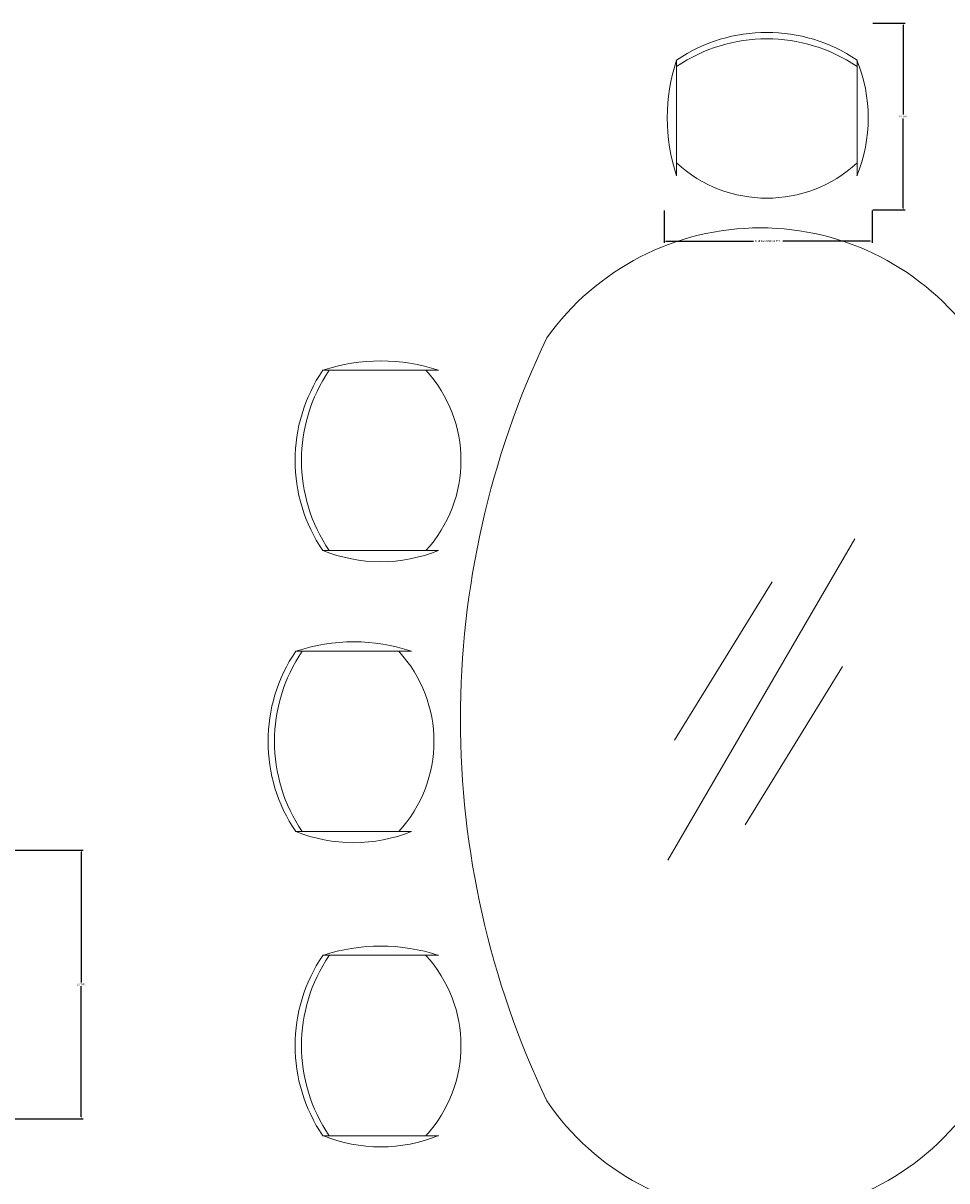
# Model space of a CAD drawing. Units: inches. Extents: x -61 to 1599, y -1316 to 257.
# Tile 169 of 204: x 1214 to 1304, y -937 to -825. Entities that reach past the tile are written whole.
import ezdxf

# ---------------------------------------------------------------- set-up
doc = ezdxf.new("R2010")
doc.units = ezdxf.units.IN
doc.header["$MEASUREMENT"] = 0
doc.layers.add('A-ANNO-DIMS', color=2, linetype='Continuous', lineweight=18)
doc.layers.add('FURNITURE', color=83, linetype='Continuous', lineweight=18)
doc.styles.get("Standard").update_dxf_attribs({"font": 'arial.ttf'})
doc.dimstyles.get("Standard").update_dxf_attribs({"dimtxt": 0.18, "dimasz": 0.18, "dimexe": 0.18, "dimexo": 0.0625, "dimgap": 0.09, "dimtad": 0, "dimtih": 1, "dimtoh": 1, "dimdec": 0, "dimzin": 0, "dimdsep": 46, "dimlunit": 3, "dimtxsty": 'Standard', "dimcen": 0.09, "dimadec": 0, "dimazin": 0, "dimtfac": 1, "dimtdec": 0, "dimtofl": 0, "dimtmove": 0, "dimatfit": 3, "dimfxl": 1, "dimtolj": 1, "dimtzin": 0, "dimarcsym": 0})

# ---------------------------------------------------------------- blocks, each defined once
blk = doc.blocks.new('DINING-TABLE-OVAL')
for p, q in [((20.06, 34.26), (38.12, 65.35)), ((20.69, 45.86), (30.12, 61.18)), ((27.51, 37.68), (36.94, 53.01))]:
    blk.add_line(p, q)
for centre, radius, start, end in [((28.99, 70.07), 25.36, 35.5172, 144.4828), ((85.79, 47.89), 85.79, 154.5151, 205.4849), ((-21.85, 47.89), 80.45, 332.689, 27.311), ((28.99, 24.89), 24.89, 213.9753, 326.0247)]:
    blk.add_arc(centre, radius, start, end)
blk = doc.blocks.new('DINING-CHAIR')
for p, q in [((0.9, 2.16), (0.9, 13.35)), ((18.35, 2.16), (18.35, 13.35))]:
    blk.add_line(p, q)
for centre, radius, start, end in [((9.63, 0.52), 15.52, 55.8098, 124.1902), ((9.63, -0.1), 15.52, 55.8098, 124.1902), ((17.78, 7.76), 17.78, 161.6455, 198.3545), ((4.51, 7.76), 14.92, 337.9646, 22.0354), ((9.63, 12.87), 12.87, 227.332, 312.668)]:
    blk.add_arc(centre, radius, start, end)
blk = doc.blocks.new('*D612')
at = {"layer": 'A-ANNO-DIMS', "color": 0, "lineweight": -2, "transparency": 16777216}
for p, q in [((1276.32, -843.37), (1276.32, -846.5)), ((1296.42, -843.37), (1296.42, -846.5)), ((1276.5, -846.32), (1284.95, -846.32)), ((1296.24, -846.32), (1287.8, -846.32))]:
    blk.add_line(p, q, dxfattribs=at)
at = {"layer": 'A-ANNO-DIMS', "color": 0, "transparency": 16777216}
for points in [[(1276.5, -846.29), (1276.5, -846.35), (1276.32, -846.32)], [(1296.24, -846.29), (1296.24, -846.35), (1296.42, -846.32)]]:
    blk.add_solid(points, dxfattribs=at)
at = {"layer": 'DEFPOINTS', "color": 0, "transparency": 16777216}
for p in [(1276.32, -843.31), (1296.42, -843.31), (1296.42, -846.32)]:
    blk.add_point(p, dxfattribs=at)
at = {"layer": 'A-ANNO-DIMS', "color": 0, "transparency": 16777216, "insert": (1286.37, -846.32), "char_height": 0.18, "attachment_point": 5}
blk.add_mtext('\\A1;DINING CHAIR 20 TYP.', dxfattribs=at)
blk = doc.blocks.new('*D613')
at = {"layer": 'A-ANNO-DIMS', "color": 0, "lineweight": -2, "transparency": 16777216}
for p, q in [((1296.49, -825.24), (1299.62, -825.24)), ((1299.44, -825.42), (1299.44, -834.09)), ((1299.44, -843.13), (1299.44, -834.45)), ((1296.49, -843.31), (1299.62, -843.31))]:
    blk.add_line(p, q, dxfattribs=at)
at = {"layer": 'A-ANNO-DIMS', "color": 0, "transparency": 16777216}
for points in [[(1299.41, -825.42), (1299.47, -825.42), (1299.44, -825.24)], [(1299.41, -843.13), (1299.47, -843.13), (1299.44, -843.31)]]:
    blk.add_solid(points, dxfattribs=at)
at = {"layer": 'DEFPOINTS', "color": 0, "transparency": 16777216}
for p in [(1296.42, -825.24), (1299.44, -825.24), (1296.42, -843.31)]:
    blk.add_point(p, dxfattribs=at)
at = {"layer": 'A-ANNO-DIMS', "color": 0, "transparency": 16777216, "insert": (1299.44, -834.27), "char_height": 0.18, "attachment_point": 5}
blk.add_mtext('\\A1;18 TYP.', dxfattribs=at)
blk = doc.blocks.new('*D685')
at = {"layer": 'A-ANNO-DIMS', "color": 0, "lineweight": -2, "transparency": 16777216}
for p, q in [((1207.44, -905.23), (1220.15, -905.23)), ((1219.97, -905.41), (1219.97, -918.04)), ((1219.97, -931.05), (1219.97, -918.41)), ((1207.44, -931.23), (1220.15, -931.23))]:
    blk.add_line(p, q, dxfattribs=at)
at = {"layer": 'A-ANNO-DIMS', "color": 0, "transparency": 16777216}
for points in [[(1219.94, -905.41), (1220, -905.41), (1219.97, -905.23)], [(1219.94, -931.05), (1220, -931.05), (1219.97, -931.23)]]:
    blk.add_solid(points, dxfattribs=at)
at = {"layer": 'DEFPOINTS', "color": 0, "transparency": 16777216}
for p in [(1207.37, -905.23), (1219.97, -905.23), (1207.37, -931.23)]:
    blk.add_point(p, dxfattribs=at)
at = {"layer": 'A-ANNO-DIMS', "color": 0, "transparency": 16777216, "insert": (1219.97, -918.23), "char_height": 0.18, "attachment_point": 5}
blk.add_mtext('\\A1;26 TYP.', dxfattribs=at)

msp = doc.modelspace()

# ---------------------------------------------------------------- block references
at = {"layer": 'FURNITURE'}
for name, p in [('DINING-CHAIR', (1276.622, -842.1701)), ('DINING-TABLE-OVAL', (1256.634, -940.4721))]:
    msp.add_blockref(name, p, dxfattribs=at)
at = {"layer": 'FURNITURE', "extrusion": (0, 0, -1), "zscale": -1}
for p, rotation in [((-1256.681, -857.909), 269.9999999999993), ((-1254.0669, -885.0906), 269.9999999999979), ((-1256.681, -914.5159), 269.9999999999997)]:
    msp.add_blockref('DINING-CHAIR', p, dxfattribs=dict(at, rotation=rotation))

# ---------------------------------------------------------------- dimensions: what is measured, and where the dimension line sits
at = {"layer": 'A-ANNO-DIMS'}
for base, p1, p2, picture, middle in [((1299.4386, -825.2394), (1296.4232, -843.3051), (1296.4232, -825.2394), '*D613', (1299.4386, -834.2723)), ((1219.9746, -905.2253), (1207.3746, -931.2253), (1207.3746, -905.2253), '*D685', (1219.9746, -918.2253))]:
    dim = msp.add_linear_dim(base=base, p1=p1, p2=p2, angle=90, text='<> TYP.', dimstyle='Standard', override={"dimdec": 0, "dimlfac": 1, "dimrnd": 0, "dimzin": 0, "dimdsep": 46, "dimlunit": 2}, dxfattribs=at)
    dim.commit()
    dim.dimension.update_dxf_attribs({"geometry": picture, "text_midpoint": middle})
dim = msp.add_linear_dim(base=(1296.4232, -846.3204), p1=(1276.3209, -843.3051), p2=(1296.4232, -843.3051), text='DINING CHAIR <> TYP.', dimstyle='Standard', override={"dimdec": 0, "dimlfac": 1, "dimrnd": 0, "dimzin": 0, "dimdsep": 46, "dimlunit": 2}, dxfattribs=at)
dim.commit()
dim.dimension.update_dxf_attribs({"geometry": '*D612', "text_midpoint": (1286.3721, -846.3204)})

doc.saveas('drawing.dxf')
